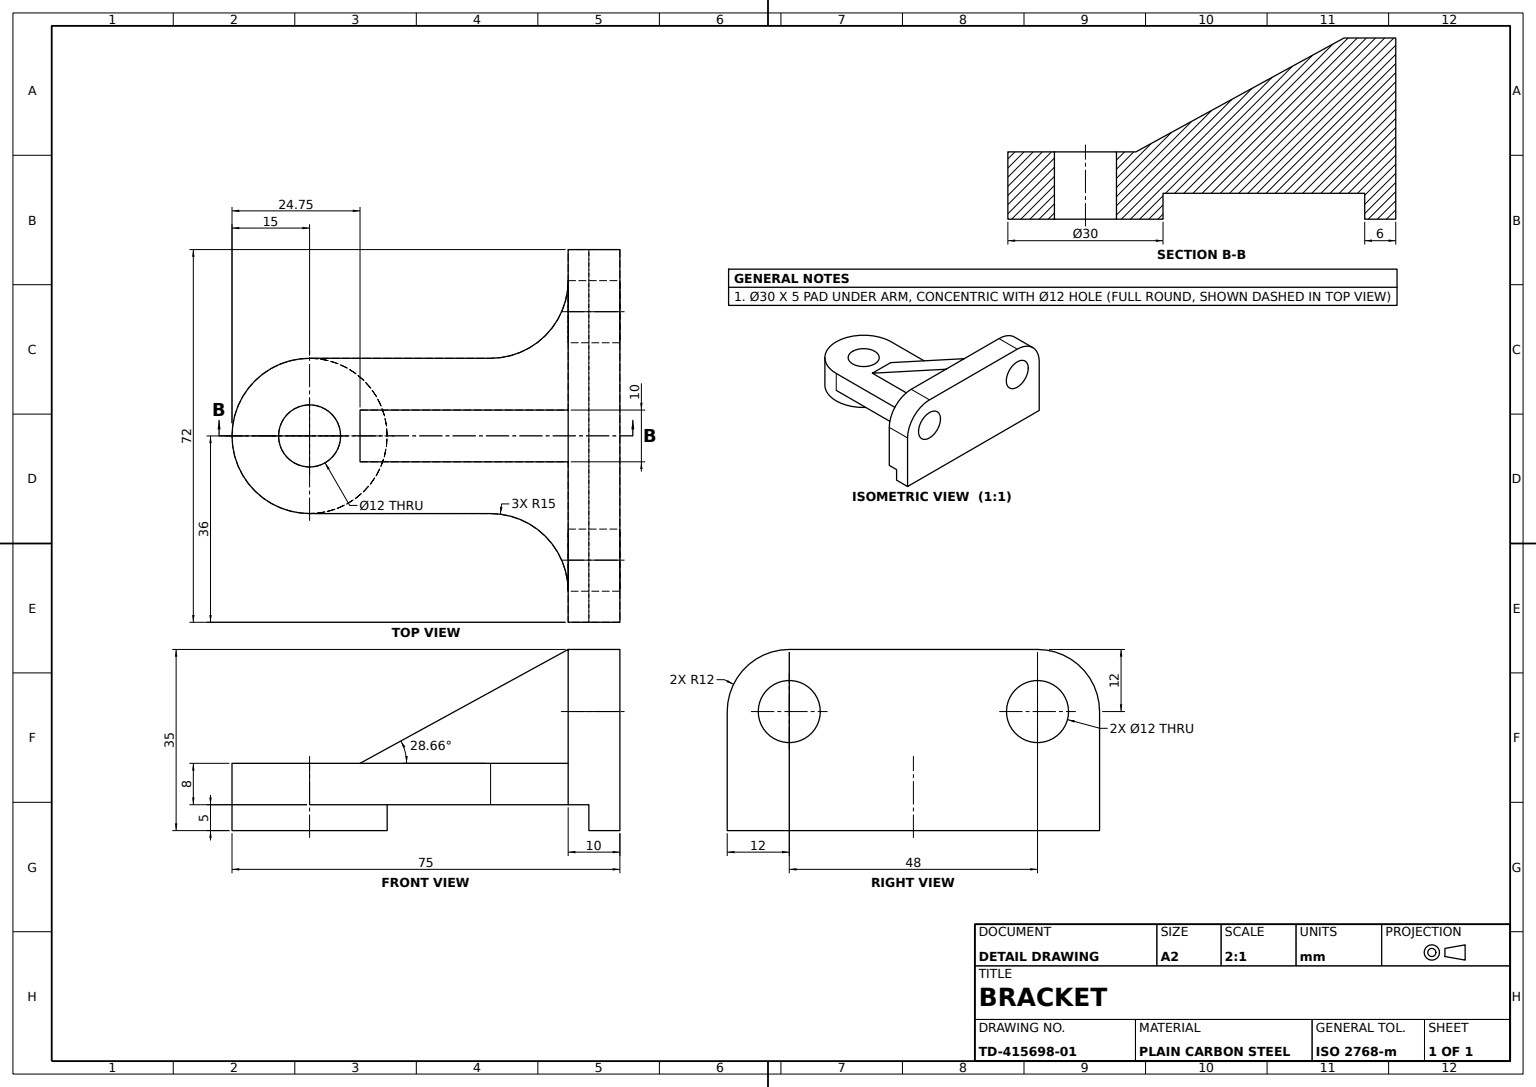
SolidWorks part; units mm, degrees
material "Plain Carbon Steel"
ref_plane "Front Plane" through (0, 0, 0) normal (0, 0, 1) x (1, 0, 0)
ref_plane "Top Plane" through (0, 0, 0) normal (0, 1, 0) x (1, 0, 0)
ref_plane "Right Plane" through (0, 0, 0) normal (1, 0, 0) x (0, 0, -1)
sketch "Plate Profile Sketch" plane through (0, 0, 0) normal (0, 0, 1) x (1, 0, 0)
  line L0 (0, 0) -> (0, -23)
  line L1 (0, -23) -> (72, -23)
  line L2 (72, -23) -> (72, 0)
  line L5 (12, 12) -> (60, 12)
  arc A0 (12, 12) -> (0, 0) centre (12, 0) ccw
  arc A1 (72, 0) -> (60, 12) centre (60, 0) ccw
  dimension "D1" = 24
  dimension "D2" = 24
  dimension "D3" = 12
  dimension "D4" = 72
  dimension "D5" = 35
extrude "Mounting Plate" add sketch "Plate Profile Sketch" along normal blind 10
sketch "Plate Notch Sketch" plane through (0, 0, 0) normal (-1, 0, 0) x (0, 0, 1)
  line L0 (0, 0) -> (0, -23) construction
  line L1 (10, -23) -> (0, -23) construction
  line L2 (6, -23) -> (6, -18)
  line L3 (6, -18) -> (10, -18)
  line L4 (10, 0) -> (10, -23) construction
  line L5 (10, -18) -> (10, -23)
  line L6 (10, -23) -> (6, -23)
  dimension "D1" = 6
  dimension "D2" = 5
extrude "Plate Notch Cut" cut sketch "Plate Notch Sketch" against normal blind 72
sketch "Arm Profile Sketch" plane through (0, -18, 0) normal (0, -1, 0) x (1, 0, 0)
  line L0 (6, 10) -> (66, 10)
  line L1 (72, 10) -> (0, 10) construction
  line L2 (21, 60) -> (21, 25)
  line L4 (51, 60) -> (51, 25)
  arc A0 (51, 60) -> (21, 60) centre (36, 60) ccw
  arc A1 (51, 25) -> (66, 10) centre (66, 25) ccw
  arc A2 (21, 25) -> (6, 10) centre (6, 25) cw
  point P14 (51, 10)
  point P17 (21, 10)
  dimension "D1" = 30
  dimension "D2" = 15
  dimension "D3" = 15
  dimension "D4" = 36
  dimension "D5" = 60
  dimension "D6" = 35
extrude "Pivot Arm" add sketch "Arm Profile Sketch" against normal blind 8
sketch "Pivot Boss Sketch" plane through (0, -18, 0) normal (0, -1, 0) x (1, 0, 0)
  circle A0 centre (36, 60) radius 15
  dimension "D1" = 30
  dimension "D2" = 30
extrude "Pivot Boss Ø30" add sketch "Pivot Boss Sketch" along normal blind 5
sketch "Plate Holes Sketch" plane through (0, 0, 10) normal (0, 0, 1) x (1, 0, 0)
  circle A0 centre (12, 0) radius 6
  circle A1 centre (60, 0) radius 6
  dimension "D1" = 12
  dimension "D2" = 12
  dimension "D3" = 12
extrude "Plate Holes 2xØ12" cut sketch "Plate Holes Sketch" against normal blind 10
sketch "Pivot Hole Sketch" plane through (0, -23, 0) normal (0, -1, 0) x (1, 0, 0)
  circle A0 centre (36, 60) radius 6
  dimension "D1" = 12
  dimension "D2" = 12
extrude "Pivot Hole Ø12" cut sketch "Pivot Hole Sketch" against normal blind 13
sketch "Gusset Profile Sketch" plane through (0, 0, 0) normal (-1, 0, 0) x (0, 0, 1)
  line L0 (10, -10) -> (50.2459, -10)
  line L1 (60, -10) -> (25, -10) construction
  line L2 (50.2459, -10) -> (10, 12)
  line L3 (10, 12) -> (10, -10)
  line L4 (6, -18) -> (6, -23) construction
  dimension "D1" = 44.2459
extrude "Gusset Blank" add sketch "Gusset Profile Sketch" against normal blind 42
sketch "Gusset Taper Sketch" plane through (0, 0, 0) normal (-1, 0, 0) x (0, 0, 1)
  line L0 (10, 12) -> (10, -10)
  line L1 (10, -10) -> (50.2459, -10)
  line L2 (50.2459, -10) -> (10, 12)
extrude "Gusset Taper Cut" cut sketch "Gusset Taper Sketch" against normal blind 30
sketch "Gusset Edge Trim A Sketch" plane through (30, 0, 0) normal (-1, 0, 0) x (0, 0, 1)
  line L0 (10, 12) -> (10, -10)
  line L1 (10, -10) -> (50.2459, -10)
  line L2 (50.2459, -10) -> (10, 12)
extrude "Gusset Edge Trim A" cut sketch "Gusset Edge Trim A Sketch" against normal blind 1
sketch "Gusset Edge Trim B Sketch" plane through (42, 0, 0) normal (1, 0, 0) x (0, 0, -1)
  line L0 (-50.2459, -10) -> (-10, -10)
  line L1 (-10, -10) -> (-10, 12)
  line L2 (-10, 12) -> (-50.2459, -10)
extrude "Gusset Edge Trim B" cut sketch "Gusset Edge Trim B Sketch" against normal blind 1
